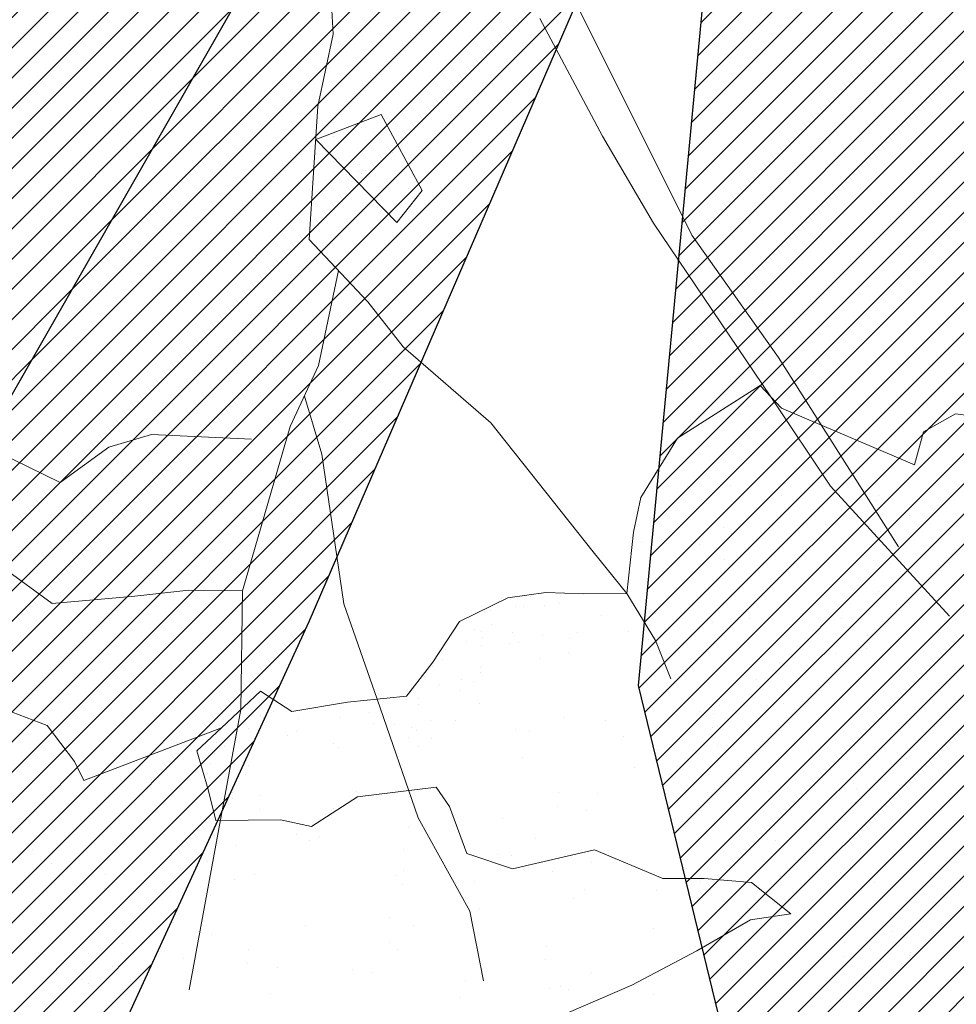
# Model space of a CAD drawing. Units: inches. Extents: x 1986 to 21484, y -1816 to 2016.
# Tile 65 of 85: x 3662.33 to 3669.081, y 1870.798 to 1877.893. Entities that reach past the tile are written whole.
import ezdxf

# ---------------------------------------------------------------- set-up
doc = ezdxf.new("R2010")
doc.units = ezdxf.units.IN
doc.layers.add('L-PLNT', color=84, linetype='Continuous', lineweight=13)
doc.layers.add('vfolhas', color=114, linetype='Continuous', lineweight=5)
for name, color, linetype in [('vfolha', 72, 'Continuous'), ('vfolha2', 110, 'Continuous'), ('vfolhas2', 102, 'Continuous')]:
    doc.layers.add(name, color=color, linetype=linetype)
pattern_1 = [(45, (-2446.5133113, 50.986076), (-0.004419417382, 0.004419417382), [])]

# ---------------------------------------------------------------- blocks, each defined once
blk = doc.blocks.new('arbusto_PB_verde_grande')
at = {"layer": 'vfolha2'}
h = blk.add_hatch(dxfattribs=at)
h.set_pattern_fill('ANSI31', color=256, scale=0.05, style=0)
h.set_pattern_definition(pattern_1)
h.paths.add_polyline_path([(0.02944, 0.35651), (0.00028, 0.09048), (0.02625, -0.03934), (0.047, 0.06233), (0.06189, 0.09731), (0.09372, 0.26573), (0.09955, 0.43473), (0.08789, 0.61313), (0.0645, 0.72266), (0.04988, 0.6851), (0.0236, 0.51294)])
h.paths.add_polyline_path([(0.30106, 0.43789), (0.14225, 0.24871), (0.26685, 0.30022)])
h.paths.add_polyline_path([(0.37995, 0.22817), (0.23697, 0.15193), (0.18428, 0.09364), (0.11122, 0.04358), (0.02625, -0.03934), (0.28061, 0.04667), (0.36829, 0.07798), (0.46756, 0.11239), (0.61068, 0.19376), (0.71585, 0.27823), (0.55813, 0.25948)])
h.paths.add_polyline_path([(0.56101, -0.29441), (0.72752, -0.32573), (0.59024, -0.2412), (0.42962, -0.15982), (0.02625, -0.03934), (0.14922, -0.14107), (0.18838, -0.16604), (0.41501, -0.24435)])
h.paths.add_polyline_path([(-0.27429, -0.44776), (-0.30352, -0.72628), (-0.23923, -0.64175), (-0.15457, -0.45716), (0.02625, -0.03934), (-0.16328, -0.25376)])
h.paths.add_polyline_path([(-0.51963, -0.24744), (-0.67736, -0.32573), (-0.59558, -0.35072), (-0.40574, -0.32882), (-0.21007, -0.20995), (0.02625, -0.03934), (-0.14874, -0.06595), (-0.31518, -0.09101), (-0.41452, -0.15048)])
h.paths.add_polyline_path([(-0.52546, 0.25007), (-0.70947, 0.24698), (-0.51963, 0.1093), (-0.32979, 0.02167), (-0.07567, -0.0128), (-0.04234, -0.02148), (-0.35024, 0.1312)])
at = {"layer": 'vfolhas'}
h = blk.add_hatch(dxfattribs=at)
h.set_pattern_fill('ANSI31', color=256, scale=0.05, style=0)
h.set_pattern_definition(pattern_1)
h.paths.add_polyline_path([(-0.07279, 0.50669), (-0.18085, 0.65063), (-0.2334, 0.67253), (-0.20712, 0.53176), (-0.10785, 0.25007), (0.02625, -0.03934), (0.00028, 0.09048), (0.00816, 0.16241), (-0.04939, 0.29079)])
h.paths.add_polyline_path([(0.09902, 0.41929), (0.09372, 0.26573), (0.07906, 0.18814), (0.15506, 0.36901), (0.26606, 0.5505), (0.28356, 0.63504), (0.2485, 0.68819), (0.25145, 0.63504), (0.20178, 0.54426)])
h.paths.add_polyline_path([(0.12295, 0.24073), (0.047, 0.06233), (0.02625, -0.03934), (0.11122, 0.04358), (0.18428, 0.09364), (0.27478, 0.19376), (0.3215, 0.25323), (0.44129, 0.38467), (0.47634, 0.57866), (0.41789, 0.45347), (0.28939, 0.30954)])
h.paths.add_polyline_path([(0.58145, -0.03779), (0.70707, 0.01536), (0.78591, 0.04667), (0.74796, 0.06549), (0.62818, 0.08423), (0.52595, 0.09048), (0.39745, 0.04358), (0.02625, -0.03934), (0.25728, -0.03154), (0.43834, -0.0347)])
h.paths.add_polyline_path([(0.52022, -0.03647), (0.43834, -0.0347), (0.25728, -0.03154), (0.02625, -0.03934), (0.17964, -0.08515), (0.53768, -0.13167), (0.69541, -0.15357), (0.78591, -0.07852), (0.70413, -0.10042)])
h.paths.add_polyline_path([(0.27189, -0.21929), (0.14922, -0.14107), (0.02625, -0.03934), (0.15794, -0.31007), (0.29522, -0.42585), (0.41789, -0.49157), (0.56396, -0.56669), (0.5114, -0.48532), (0.39456, -0.34139)])
h.paths.add_polyline_path([(-0.05818, -0.47591), (-0.02312, -0.61984), (0.047, -0.80134), (0.08494, -0.59794), (0.07911, -0.4071), (0.03527, -0.25376), (0.02625, -0.03934), (-0.03773, -0.26001)])
h.paths.add_polyline_path([(-0.24218, 0.14054), (-0.11073, 0.06858), (0.02625, -0.03934), (-0.04235, 0.10871), (-0.21007, 0.23757), (-0.36485, 0.33145), (-0.47874, 0.40341), (-0.54303, 0.46288), (-0.49041, 0.33145), (-0.39408, 0.22192)])
h = blk.add_hatch(dxfattribs=at)
h.set_pattern_fill('ANSI31', color=256, scale=0.05, style=0)
h.set_pattern_definition(pattern_1)
h.paths.add_polyline_path([(-0.57219, 0.06233), (-0.7153, 0.10298), (-0.67736, 0.08107), (-0.62769, 0.01536), (-0.56347, -0.04095), (-0.26461, -0.0834), (-0.14874, -0.06595), (-0.10151, -0.05877), (-0.20418, -0.0472), (-0.40279, -0.00339)])
h.paths.add_polyline_path([(-0.56347, -0.04095), (-0.58279, -0.02401), (-0.72992, -0.09726), (-0.4334, -0.1679), (-0.41452, -0.15048), (-0.31518, -0.09101), (-0.26461, -0.0834)])
h.paths.add_polyline_path([(-0.2769, -0.47267), (-0.27429, -0.44776), (-0.16328, -0.25376), (0.02625, -0.03934), (-0.21007, -0.20995), (-0.2672, -0.24466), (-0.36485, -0.35697), (-0.42907, -0.46341), (-0.47586, -0.60425), (-0.37946, -0.57603)])
at = {"layer": 'vfolha'}
blk.add_line((-0.03773, -0.26001), (-0.05818, -0.47591), dxfattribs=at)
at = {"layer": 'vfolha2'}
for p, q in [((-0.15457, -0.45716), (0.02625, -0.03934)), ((-0.16328, -0.25376), (-0.27429, -0.44776))]:
    blk.add_line(p, q, dxfattribs=at)
at = {"layer": 'vfolhas2'}
for p, q in [((-0.23923, -0.64175), (-0.15457, -0.45716)), ((-0.05818, -0.47591), (-0.02312, -0.61984))]:
    blk.add_line(p, q, dxfattribs=at)
blk = doc.blocks.new('PLANT-SHRUB')
for p, q in [((2172.8941, 1899.1254), (2172.8941, 1899.1254)), ((2172.3465, 1898.9991), (2172.3465, 1898.9991)), ((2172.8894, 1898.9276), (2172.8894, 1898.9276)), ((2173.0974, 1898.9002), (2173.0974, 1898.9002)), ((2173.2665, 1898.8143), (2173.2665, 1898.8143)), ((2173.4223, 1898.8574), (2173.4223, 1898.8574)), ((2172.387, 1898.7252), (2172.387, 1898.7252)), ((2173.1929, 1898.7468), (2173.1929, 1898.7468)), ((2173.4331, 1898.7118), (2173.4331, 1898.7118)), ((2172.7402, 1898.579), (2172.7402, 1898.579)), ((2173.9848, 1898.5768), (2173.9848, 1898.5768)), ((2172.7951, 1898.3823), (2172.7951, 1898.3823)), ((2171.8465, 1898.3504), (2171.8465, 1898.3504)), ((2172.8689, 1898.3554), (2172.8689, 1898.3554)), ((2173.3353, 1898.3284), (2173.3864, 1897.9709)), ((2173.3353, 1898.3284), (2173.3353, 1898.3284)), ((2173.5781, 1898.1624), (2173.3353, 1898.3284)), ((2173.9484, 1898.3165), (2173.9484, 1898.3165)), ((2172.1334, 1898.1925), (2172.1334, 1898.1925)), ((2173.3781, 1898.1902), (2173.3781, 1898.1902)), ((2174.0125, 1898.0603), (2173.5781, 1898.1624)), ((2171.9649, 1898.0851), (2171.9649, 1898.0851)), ((2171.6531, 1898.0555), (2171.6531, 1898.0555)), ((2171.978, 1898.0128), (2171.978, 1898.0128)), ((2172.4473, 1898.0636), (2172.4473, 1898.0636)), ((2173.2095, 1898.0828), (2173.2095, 1898.0828)), ((2173.9965, 1898.0315), (2173.9965, 1898.0315)), ((2174.5236, 1897.9199), (2174.0125, 1898.0603)), ((2174.4542, 1898.0806), (2174.4542, 1898.0806)), ((2172.3618, 1897.9551), (2172.3618, 1897.9551)), ((2172.3737, 1897.9961), (2172.3737, 1897.9961)), ((2173.3864, 1897.9709), (2173.6164, 1897.7156)), ((2173.408, 1897.9417), (2173.408, 1897.9417)), ((2174.4304, 1897.9466), (2174.4304, 1897.9466)), ((2172.5209, 1897.9413), (2172.5209, 1897.9413)), ((2172.7289, 1897.9139), (2172.7289, 1897.9139)), ((2173.0538, 1897.8711), (2173.0538, 1897.8711)), ((2175.2263, 1897.6645), (2174.5236, 1897.9199)), ((2173.5967, 1897.7997), (2173.5967, 1897.7997)), ((2173.8047, 1897.7723), (2173.8047, 1897.7723)), ((2174.1296, 1897.7295), (2174.1296, 1897.7295)), ((2173.6164, 1897.7156), (2173.8336, 1897.5113)), ((2173.6488, 1897.7129), (2173.6488, 1897.7129)), ((2174.6725, 1897.658), (2174.6725, 1897.658)), ((2171.9759, 1897.6316), (2171.9759, 1897.6316)), ((2173.5751, 1897.6454), (2173.5751, 1897.6454)), ((2174.8805, 1897.6306), (2174.8805, 1897.6306)), ((2171.0333, 1897.5479), (2171.0183, 1896.2787)), ((2171.1728, 1897.5805), (2171.1728, 1897.5805)), ((2171.8213, 1897.5804), (2171.8213, 1897.5804)), ((2172.4174, 1897.5782), (2172.4174, 1897.5782)), ((2172.8437, 1897.5853), (2172.8437, 1897.5853)), ((2173.662, 1897.5759), (2173.662, 1897.5759)), ((2173.9232, 1897.5464), (2173.9232, 1897.5464)), ((2174.9067, 1897.5737), (2174.9067, 1897.5737)), ((2174.9694, 1897.533), (2174.9694, 1897.533)), ((2173.8336, 1897.5113), (2174.0508, 1897.0262)), ((2171.6282, 1897.313), (2171.6282, 1897.313)), ((2174.8503, 1897.3621), (2174.8503, 1897.3621)), ((2171.5545, 1897.2455), (2171.5545, 1897.2455)), ((2173.1773, 1897.2808), (2173.1773, 1897.2808)), ((2174.7766, 1897.2946), (2174.7766, 1897.2946)), ((2171.2571, 1897.2239), (2171.2571, 1897.2239)), ((2171.8106, 1897.1917), (2171.8106, 1897.1917)), ((2172.3366, 1897.185), (2172.3366, 1897.185)), ((2173.0553, 1897.1894), (2173.0553, 1897.1894)), ((2173.3828, 1897.1716), (2173.3828, 1897.1716)), ((2174.2999, 1897.1871), (2174.2999, 1897.1871)), ((2174.4052, 1897.1765), (2174.4052, 1897.1765)), ((2175.0099, 1896.7314), (2175.2812, 1897.1651)), ((2171.0765, 1897.0966), (2171.0765, 1897.0966)), ((2175.4846, 1897.1377), (2175.4846, 1897.1377)), ((2171.2846, 1897.0692), (2171.2846, 1897.0692)), ((2171.6095, 1897.0265), (2171.6095, 1897.0265)), ((2171.6421, 1897.0843), (2171.6421, 1897.0843)), ((2172.8867, 1897.082), (2172.8867, 1897.082)), ((2174.0508, 1897.0262), (2174.5747, 1896.7198)), ((2174.1314, 1897.0798), (2174.1314, 1897.0798)), ((2175.376, 1897.0775), (2175.376, 1897.0775)), ((2172.1524, 1896.955), (2172.1524, 1896.955)), ((2172.8296, 1896.9622), (2172.8296, 1896.9622)), ((2170.6548, 1895.3462), (2170.9596, 1896.9325)), ((2171.1567, 1896.881), (2171.1567, 1896.881)), ((2172.3604, 1896.9276), (2172.3604, 1896.9276)), ((2172.6853, 1896.8848), (2172.6853, 1896.8848)), ((2172.756, 1896.8947), (2172.756, 1896.8947)), ((2174.3788, 1896.9301), (2174.3788, 1896.9301)), ((2170.0023, 1896.5154), (2169.7439, 1896.8381)), ((2170.75, 1896.8236), (2170.75, 1896.8236)), ((2171.7962, 1896.8103), (2171.7962, 1896.8103)), ((2172.8186, 1896.8152), (2172.8186, 1896.8152)), ((2173.2282, 1896.8134), (2173.2282, 1896.8134)), ((2173.4362, 1896.786), (2173.4362, 1896.786)), ((2173.7612, 1896.7432), (2173.7612, 1896.7432)), ((2173.898, 1896.7763), (2173.898, 1896.7763)), ((2174.9442, 1896.7629), (2174.9442, 1896.7629)), ((2174.304, 1896.6717), (2174.304, 1896.6717)), ((2174.5747, 1896.7198), (2174.7408, 1896.4134)), ((2174.82, 1895.986), (2175.0099, 1896.7314)), ((2174.0311, 1896.6114), (2174.0311, 1896.6114)), ((2174.5121, 1896.6443), (2174.5121, 1896.6443)), ((2174.837, 1896.6016), (2174.837, 1896.6016)), ((2170.4705, 1896.58), (2170.2606, 1896.4509)), ((2170.8904, 1895.628), (2170.4705, 1896.58)), ((2170.809, 1896.5624), (2170.809, 1896.5624)), ((2170.85, 1896.5796), (2170.85, 1896.5796)), ((2172.0946, 1896.5774), (2172.0946, 1896.5774)), ((2172.3582, 1896.5302), (2172.3582, 1896.5302)), ((2173.3392, 1896.5751), (2173.3392, 1896.5751)), ((2173.9574, 1896.5439), (2173.9574, 1896.5439)), ((2174.5839, 1896.5729), (2174.5839, 1896.5729)), ((2175.3798, 1896.5301), (2175.3798, 1896.5301)), ((2175.5803, 1896.5793), (2175.5803, 1896.5793)), ((2175.8285, 1896.5706), (2175.8285, 1896.5706)), ((2170.2606, 1896.4509), (2170.0023, 1896.5154)), ((2171.232, 1896.4538), (2171.232, 1896.4538)), ((2172.6969, 1896.2259), (2172.8056, 1896.5036)), ((2175.5879, 1896.5027), (2175.5879, 1896.5027)), ((2175.9128, 1896.4599), (2175.9128, 1896.4599)), ((2172.3114, 1896.4149), (2172.3114, 1896.4149)), ((2173.3576, 1896.4015), (2173.3576, 1896.4015)), ((2174.38, 1896.4064), (2174.38, 1896.4064)), ((2174.7408, 1896.4134), (2174.6003, 1896.0814)), ((2175.4595, 1896.3676), (2175.4595, 1896.3676)), ((2171.0183, 1896.2787), (2170.8904, 1895.5151)), ((2175.2326, 1896.2607), (2175.2326, 1896.2607)), ((2171.4879, 1896.1908), (2171.4879, 1896.1908)), ((2172.0105, 1896.2116), (2172.0105, 1896.2116)), ((2172.6181, 1895.8378), (2172.6969, 1896.2259)), ((2172.7325, 1896.1886), (2172.7325, 1896.1886)), ((2173.5596, 1896.1794), (2173.5596, 1896.1794)), ((2173.9771, 1896.1863), (2173.9771, 1896.1863)), ((2175.1589, 1896.1932), (2175.1589, 1896.1932)), ((2175.2218, 1896.1841), (2175.2218, 1896.1841)), ((2176.4664, 1896.1818), (2176.4664, 1896.1818)), ((2171.9368, 1896.1441), (2171.9368, 1896.1441)), ((2170.9161, 1896.083), (2170.9161, 1896.083)), ((2171.241, 1896.0402), (2171.241, 1896.0402)), ((2171.3193, 1896.0835), (2171.3193, 1896.0835)), ((2171.771, 1896.0402), (2171.771, 1896.0402)), ((2172.564, 1896.0812), (2172.564, 1896.0812)), ((2172.7934, 1896.0451), (2172.7934, 1896.0451)), ((2173.8086, 1896.0789), (2173.8086, 1896.0789)), ((2174.6003, 1896.0814), (2174.5747, 1895.9155)), ((2175.0532, 1896.0767), (2175.0532, 1896.0767)), ((2176.2979, 1896.0744), (2176.2979, 1896.0744)), ((2171.7839, 1895.9687), (2171.7839, 1895.9687)), ((2173.8729, 1896.0062), (2173.8729, 1896.0062)), ((2174.4507, 1895.1602), (2174.82, 1895.986)), ((2174.919, 1895.9928), (2174.919, 1895.9928)), ((2175.9414, 1895.9977), (2175.9414, 1895.9977)), ((2171.9919, 1895.9413), (2171.9919, 1895.9413)), ((2172.3168, 1895.8985), (2172.3168, 1895.8985)), ((2174.5747, 1895.9155), (2175.0362, 1895.5766)), ((2176.434, 1895.9099), (2176.434, 1895.9099)), ((2172.6181, 1895.8378), (2172.279, 1895.5474)), ((2172.5881, 1895.4532), (2172.6181, 1895.8378)), ((2172.6181, 1895.8378), (2172.6181, 1895.8378)), ((2172.8441, 1895.628), (2172.6181, 1895.8378)), ((2172.8597, 1895.8271), (2172.8597, 1895.8271)), ((2173.2119, 1895.8608), (2173.2119, 1895.8608)), ((2174.7611, 1895.8286), (2174.7611, 1895.8286)), ((2176.3604, 1895.8424), (2176.3604, 1895.8424)), ((2171.539, 1895.7796), (2171.539, 1895.7796)), ((2173.0677, 1895.7997), (2173.0677, 1895.7997)), ((2173.1383, 1895.7933), (2173.1383, 1895.7933)), ((2173.3927, 1895.7569), (2173.3927, 1895.7569)), ((2175.2168, 1894.5433), (2176.8723, 1895.76)), ((2173.9355, 1895.6854), (2173.9355, 1895.6854)), ((2170.8904, 1895.4022), (2170.8904, 1895.628)), ((2172.2863, 1895.6448), (2172.2863, 1895.6448)), ((2173.0379, 1895.4344), (2172.8441, 1895.628)), ((2173.2694, 1895.6432), (2173.2694, 1895.6432)), ((2174.1436, 1895.658), (2174.1436, 1895.658)), ((2174.3548, 1895.6364), (2174.3548, 1895.6364)), ((2174.4685, 1895.6153), (2174.4685, 1895.6153)), ((2171.7718, 1895.5766), (2171.7718, 1895.5766)), ((2172.279, 1895.5474), (2172.0691, 1895.4022)), ((2173.017, 1895.5577), (2173.017, 1895.5577)), ((2173.426, 1895.5597), (2173.426, 1895.5597)), ((2173.7794, 1895.5299), (2173.7794, 1895.5299)), ((2173.8578, 1895.5441), (2173.8578, 1895.5441)), ((2174.2762, 1895.5388), (2174.2762, 1895.5388)), ((2175.0113, 1895.5438), (2175.0113, 1895.5438)), ((2175.0362, 1895.5766), (2175.424, 1895.5049)), ((2175.4343, 1895.5975), (2175.4343, 1895.5975)), ((2175.5057, 1895.5698), (2175.5057, 1895.5698)), ((2176.4805, 1895.5841), (2176.4805, 1895.5841)), ((2176.7503, 1895.5675), (2176.7503, 1895.5675)), ((2170.8904, 1895.5151), (2170.6507, 1894.022)), ((2172.9816, 1895.5232), (2172.9816, 1895.5232)), ((2173.1103, 1895.4974), (2173.1103, 1895.4974)), ((2173.412, 1895.4794), (2173.412, 1895.4794)), ((2173.4794, 1895.5223), (2173.4794, 1895.5223)), ((2173.75, 1895.5029), (2173.75, 1895.5029)), ((2173.9099, 1895.4785), (2173.9099, 1895.4785)), ((2173.9773, 1895.5214), (2173.9773, 1895.5214)), ((2174.3991, 1895.517), (2174.3991, 1895.517)), ((2174.4077, 1895.4776), (2174.4077, 1895.4776)), ((2174.4751, 1895.5205), (2174.4751, 1895.5205)), ((2175.2194, 1895.5164), (2175.2194, 1895.5164)), ((2175.424, 1895.5049), (2175.5533, 1895.3183)), ((2175.5443, 1895.4736), (2175.5443, 1895.4736)), ((2175.9626, 1895.4779), (2175.9626, 1895.4779)), ((2171.5847, 1895.2731), (2170.8904, 1895.4022)), ((2172.0691, 1895.4022), (2171.5847, 1895.2731)), ((2172.4915, 1894.2699), (2172.5881, 1895.4532)), ((2173.2639, 1895.2731), (2173.0379, 1895.4344)), ((2173.2231, 1895.3996), (2173.2231, 1895.3996)), ((2173.6416, 1895.3942), (2173.6416, 1895.3942)), ((2174.0505, 1895.3962), (2174.0505, 1895.3962)), ((2174.26, 1895.3895), (2174.26, 1895.3895)), ((2176.0872, 1895.4022), (2176.0872, 1895.4022)), ((2170.5087, 1894.2757), (2170.6548, 1895.3462)), ((2173.1355, 1895.3768), (2173.1355, 1895.3768)), ((2173.2655, 1895.3597), (2173.2655, 1895.3597)), ((2173.4826, 1895.3311), (2173.4826, 1895.3311)), ((2173.5658, 1895.3202), (2173.5658, 1895.3202)), ((2173.5908, 1895.357), (2173.5908, 1895.357)), ((2174.2305, 1895.3625), (2174.2305, 1895.3625)), ((2174.4823, 1895.3806), (2174.4823, 1895.3806)), ((2175.5533, 1895.3183), (2175.898, 1895.0026)), ((2176.2952, 1895.3748), (2176.2952, 1895.3748)), ((2176.6201, 1895.332), (2176.6201, 1895.332)), ((2171.5847, 1895.2731), (2171.5847, 1895.2731)), ((2173.6353, 1895.1602), (2173.2639, 1895.2731)), ((2173.4159, 1895.2516), (2173.4159, 1895.2516)), ((2173.593, 1895.2766), (2173.593, 1895.2766)), ((2173.6958, 1895.3031), (2173.6958, 1895.3031)), ((2173.9129, 1895.2745), (2173.9129, 1895.2745)), ((2174.2812, 1895.2892), (2173.9744, 1895.2408)), ((2173.9962, 1895.2635), (2173.9962, 1895.2635)), ((2174.0909, 1895.2757), (2174.0909, 1895.2757)), ((2174.2812, 1895.2892), (2174.2812, 1895.2892)), ((2174.6203, 1895.0311), (2174.2812, 1895.2892)), ((2174.5887, 1895.2748), (2174.5887, 1895.2748)), ((2177.163, 1895.2605), (2177.163, 1895.2605)), ((2173.4518, 1895.2296), (2173.4518, 1895.2296)), ((2173.9744, 1895.2408), (2173.6353, 1895.1602)), ((2173.8477, 1895.2361), (2173.8477, 1895.2361)), ((2173.9744, 1895.2408), (2173.9744, 1895.2408)), ((2174.4265, 1895.2069), (2174.4265, 1895.2069)), ((2174.5565, 1895.1898), (2174.5565, 1895.1898)), ((2174.8939, 1895.2227), (2174.8939, 1895.2227)), ((2174.899, 1895.1832), (2174.899, 1895.1832)), ((2175.9163, 1895.2276), (2175.9163, 1895.2276)), ((2176.1436, 1895.181), (2176.1436, 1895.181)), ((2176.9957, 1895.1887), (2176.9957, 1895.1887)), ((2177.371, 1895.2331), (2177.371, 1895.2331)), ((2177.3882, 1895.1787), (2177.3882, 1895.1787)), ((2174.1554, 1894.4952), (2174.4507, 1895.1602)), ((2175.6148, 1895.1592), (2175.6148, 1895.1592)), ((2177.164, 1895.1271), (2177.164, 1895.1271)), ((2174.7304, 1895.0759), (2174.7304, 1895.0759)), ((2175.5412, 1895.0917), (2175.5412, 1895.0917)), ((2175.9751, 1895.0736), (2175.9751, 1895.0736)), ((2177.2197, 1895.0713), (2177.2197, 1895.0713)), ((2174.9593, 1894.8052), (2174.6203, 1895.0311)), ((2175.7018, 1894.9686), (2175.7018, 1894.9686)), ((2175.898, 1895.0026), (2175.7831, 1894.8016)), ((2175.8474, 1895.0198), (2175.8474, 1895.0198)), ((2175.0326, 1894.9361), (2175.0326, 1894.9361)), ((2175.0968, 1894.9091), (2175.0968, 1894.9091)), ((2175.5153, 1894.9038), (2175.5153, 1894.9038)), ((2175.6723, 1894.9416), (2175.6723, 1894.9416)), ((2174.9575, 1894.8736), (2174.9575, 1894.8736)), ((2175.4553, 1894.8727), (2175.4553, 1894.8727)), ((2175.0239, 1894.5433), (2174.9593, 1894.8052)), ((2175.2896, 1894.7612), (2175.2896, 1894.7612)), ((2175.5132, 1894.7958), (2175.5132, 1894.7958)), ((2175.7831, 1894.8016), (2175.6538, 1894.5433)), ((2176.4553, 1894.814), (2176.4553, 1894.814)), ((2176.8163, 1894.8085), (2176.8163, 1894.8085)), ((2177.4777, 1894.8189), (2177.4777, 1894.8189)), ((2175.0565, 1894.71), (2175.0565, 1894.71)), ((2175.1397, 1894.6991), (2175.1397, 1894.6991)), ((2175.2126, 1894.718), (2175.2126, 1894.718)), ((2175.2697, 1894.6819), (2175.2697, 1894.6819)), ((2175.7105, 1894.7171), (2175.7105, 1894.7171)), ((2175.7214, 1894.7456), (2175.7214, 1894.7456)), ((2176.7426, 1894.741), (2176.7426, 1894.741)), ((2175.1452, 1894.6751), (2175.1452, 1894.6751)), ((2175.3446, 1894.6414), (2175.3446, 1894.6414)), ((2175.3741, 1894.6684), (2175.3741, 1894.6684)), ((2175.4869, 1894.6534), (2175.4869, 1894.6534)), ((2175.5701, 1894.6424), (2175.5701, 1894.6424)), ((2175.6431, 1894.6742), (2175.6431, 1894.6742)), ((2174.6241, 1893.928), (2175.2168, 1894.5433)), ((2175.4096, 1894.5433), (2175.0239, 1894.5433)), ((2175.0868, 1894.6011), (2175.0868, 1894.6011)), ((2175.4096, 1894.5433), (2176.393, 1894.1406)), ((2175.6538, 1894.5433), (2175.4096, 1894.5433)), ((2175.5052, 1894.5957), (2175.5052, 1894.5957)), ((2173.5315, 1893.6007), (2174.1554, 1894.4952)), ((2176.9705, 1894.4187), (2176.9705, 1894.4187)), ((2169.9359, 1892.3623), (2170.5087, 1894.2757)), ((2172.576, 1893.4368), (2172.4915, 1894.2699)), ((2177.0025, 1894.2468), (2177.0025, 1894.2468)), ((2176.393, 1894.1406), (2176.3482, 1893.9952)), ((2170.6507, 1894.022), (2170.4886, 1893.314)), ((2176.3482, 1893.9952), (2176.3146, 1893.6708)), ((2173.5633, 1893.3002), (2174.6241, 1893.928)), ((2174.904, 1893.6596), (2174.6241, 1893.928)), ((2175.2174, 1893.4246), (2174.904, 1893.6596)), ((2176.3146, 1893.6708), (2176.5609, 1893.1673)), ((2173.3379, 1893.2091), (2173.5315, 1893.6007)), ((2172.5398, 1893.0263), (2172.576, 1893.4368)), ((2175.6876, 1893.0555), (2175.2174, 1893.4246)), ((2170.4886, 1893.314), (2170.2384, 1892.3871)), ((2173.1126, 1893.1179), (2173.5633, 1893.3002)), ((2172.5398, 1892.7184), (2173.1126, 1893.1179)), ((2173.8296, 1893.1752), (2174.331, 1892.6563)), ((2175.766, 1892.6304), (2175.6876, 1893.0555)), ((2172.5398, 1892.4105), (2172.5398, 1893.0263)), ((2171.5456, 1892.1099), (2171.7066, 1892.7104)), ((2171.7066, 1892.7104), (2171.9964, 1892.7533)), ((2171.9964, 1892.7533), (2172.0126, 1891.9166)), ((2171.7643, 1892.632), (2171.7643, 1892.632)), ((2174.331, 1892.6563), (2174.6175, 1892.5132)), ((2171.68, 1892.5784), (2171.68, 1892.5784)), ((2174.6175, 1892.5132), (2175.0473, 1892.4595)), ((2171.8369, 1891.7521), (2172.5398, 1892.4105)), ((2175.0473, 1892.4595), (2175.2442, 1891.9406)), ((2171.674, 1892.3613), (2171.674, 1892.3613)), ((2171.778, 1892.3477), (2171.778, 1892.3477)), ((2171.9153, 1892.377), (2171.9153, 1892.377)), ((2171.9062, 1892.3249), (2171.9062, 1892.3249)), ((2171.9405, 1892.3263), (2171.9405, 1892.3263)), ((2171.9464, 1892.2983), (2171.9464, 1892.2983)), ((2171.6332, 1892.1988), (2171.6332, 1892.1988)), ((2171.9095, 1892.2646), (2171.9095, 1892.2646)), ((2171.6029, 1892.1316), (2171.6029, 1892.1316)), ((2171.5456, 1892.1099), (2171.5456, 1892.1099)), ((2172.0126, 1891.9166), (2171.5456, 1892.1099)), ((2171.7106, 1892.0823), (2171.7106, 1892.0823)), ((2171.9027, 1891.992), (2171.9027, 1891.992)), ((2172.0126, 1891.9166), (2172.0126, 1891.9166)), ((2171.4019, 1891.4502), (2171.8369, 1891.7521)), ((2170.979, 1890.9431), (2171.4019, 1891.4502))]:
    blk.add_line(p, q)

msp = doc.modelspace()

# ---------------------------------------------------------------- block references
at = {"layer": 'L-PLNT', "rotation": 223.1883365522388}
msp.add_blockref('PLANT-SHRUB', (3953.27, 4742.9646), dxfattribs=at)
at = {"layer": 'L-PLNT', "xscale": 24.60366729364114, "yscale": 24.60366729364114, "zscale": 24.60366729364114}
msp.add_blockref('arbusto_PB_verde_grande', (3668.2184, 1884.8051), dxfattribs=at)

doc.saveas('drawing.dxf')
